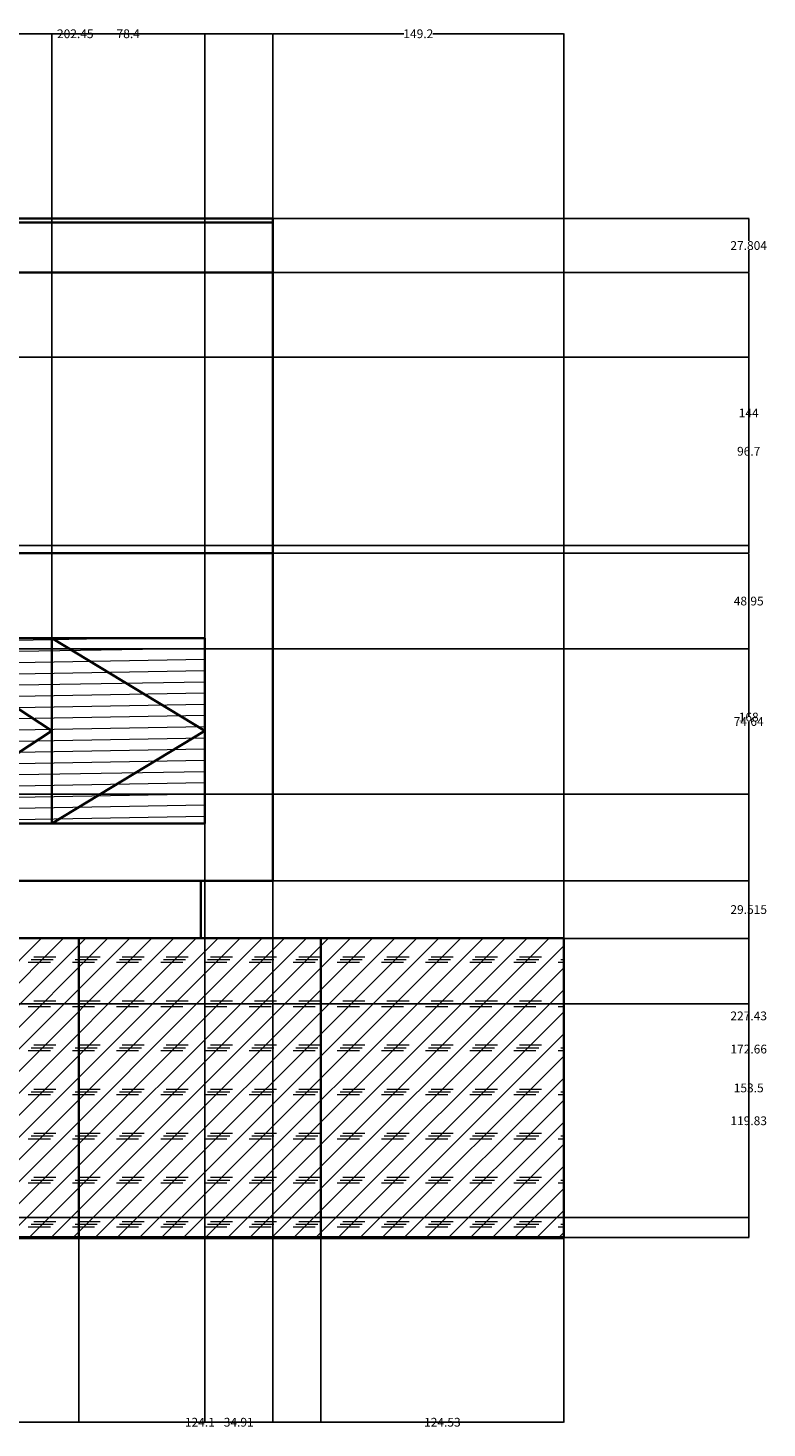
# Model space of a CAD drawing. Units: inches. Extents: x -1308 to 780, y 304 to 1023.
# Tile 7 of 7: x 402 to 780, y 304 to 1023. Entities that reach past the tile are written whole.
import ezdxf

# ---------------------------------------------------------------- set-up
doc = ezdxf.new("R2010")
doc.units = ezdxf.units.IN
doc.header["$MEASUREMENT"] = 0
for name, color, linetype, lineweight in [('A-ANNO-DIMS', 2, 'Continuous', 18), ('A-ELEV', 7, 'Continuous', 35), ('A-ELEV-GRND', 7, 'Continuous', 50), ('A-ELEV-PATT', 8, 'Continuous', 13)]:
    doc.layers.add(name, color=color, linetype=linetype, lineweight=lineweight)
doc.styles.get("Standard").update_dxf_attribs({"font": 'arial.ttf'})
doc.dimstyles.get("Standard").update_dxf_attribs({"dimtxt": 4.5, "dimasz": 0.18, "dimexe": 0.18, "dimexo": 0.0625, "dimgap": 0.09, "dimtad": 0, "dimtih": 1, "dimtoh": 1, "dimdec": 4, "dimzin": 0, "dimdsep": 46, "dimlunit": 4, "dimtxsty": 'Standard', "dimcen": 0.09, "dimadec": 0, "dimazin": 0, "dimtfac": 1, "dimtdec": 4, "dimtofl": 0, "dimtmove": 0, "dimatfit": 3, "dimfxl": 1, "dimtolj": 1, "dimtzin": 0, "dimarcsym": 0})

# ---------------------------------------------------------------- blocks, each defined once
blk = doc.blocks.new('*D1')
at = {"layer": 'A-ANNO-DIMS', "color": 0, "lineweight": -2, "transparency": 16777216}
for p, q in [((-1203.52, 401.95), (-1203.52, 307.09)), ((676.16, 401.95), (676.16, 307.09)), ((-1203.34, 307.27), (-272.9, 307.27)), ((675.98, 307.27), (-254.46, 307.27))]:
    blk.add_line(p, q, dxfattribs=at)
at = {"layer": 'A-ANNO-DIMS', "color": 0, "transparency": 16777216}
for points in [[(-1203.34, 307.3), (-1203.34, 307.24), (-1203.52, 307.27)], [(675.98, 307.3), (675.98, 307.24), (676.16, 307.27)]]:
    blk.add_solid(points, dxfattribs=at)
at = {"layer": 'Defpoints', "color": 0, "transparency": 16777216}
for p in [(-1203.52, 402.02), (676.16, 402.02), (676.16, 307.27)]:
    blk.add_point(p, dxfattribs=at)
at = {"layer": 'A-ANNO-DIMS', "color": 0, "transparency": 16777216, "insert": (-263.68, 307.27), "char_height": 4.5, "attachment_point": 5}
blk.add_mtext('\\A1;1879.7', dxfattribs=at)
blk = doc.blocks.new('*D14')
at = {"layer": 'A-ANNO-DIMS', "color": 0, "lineweight": -2, "transparency": 16777216}
for p, q in [((296.53, 555.46), (296.53, 307.09)), ((427.54, 555.46), (427.54, 307.09)), ((296.71, 307.27), (357.62, 307.27)), ((427.36, 307.27), (366.45, 307.27))]:
    blk.add_line(p, q, dxfattribs=at)
at = {"layer": 'A-ANNO-DIMS', "color": 0, "transparency": 16777216}
for points in [[(296.71, 307.3), (296.71, 307.24), (296.53, 307.27)], [(427.36, 307.3), (427.36, 307.24), (427.54, 307.27)]]:
    blk.add_solid(points, dxfattribs=at)
at = {"layer": 'Defpoints', "color": 0, "transparency": 16777216}
for p in [(296.53, 555.52), (427.54, 555.52), (427.54, 307.27)]:
    blk.add_point(p, dxfattribs=at)
at = {"layer": 'A-ANNO-DIMS', "color": 0, "transparency": 16777216, "insert": (362.03, 307.27), "char_height": 4.5, "attachment_point": 5}
blk.add_mtext('\\A1;131', dxfattribs=at)
blk = doc.blocks.new('*D15')
at = {"layer": 'A-ANNO-DIMS', "color": 0, "lineweight": -2, "transparency": 16777216}
for p, q in [((427.54, 555.46), (427.54, 307.09)), ((551.63, 555.46), (551.63, 307.09)), ((427.72, 307.27), (482.54, 307.27)), ((551.45, 307.27), (496.62, 307.27))]:
    blk.add_line(p, q, dxfattribs=at)
at = {"layer": 'A-ANNO-DIMS', "color": 0, "transparency": 16777216}
for points in [[(427.72, 307.3), (427.72, 307.24), (427.54, 307.27)], [(551.45, 307.3), (551.45, 307.24), (551.63, 307.27)]]:
    blk.add_solid(points, dxfattribs=at)
at = {"layer": 'Defpoints', "color": 0, "transparency": 16777216}
for p in [(427.54, 555.52), (551.63, 555.52), (551.63, 307.27)]:
    blk.add_point(p, dxfattribs=at)
at = {"layer": 'A-ANNO-DIMS', "color": 0, "transparency": 16777216, "insert": (489.58, 307.27), "char_height": 4.5, "attachment_point": 5}
blk.add_mtext('\\A1;124.1', dxfattribs=at)
blk = doc.blocks.new('*D16')
at = {"layer": 'A-ANNO-DIMS', "color": 0, "lineweight": -2, "transparency": 16777216}
for p, q in [((551.63, 555.46), (551.63, 307.09)), ((676.16, 555.46), (676.16, 307.09)), ((551.81, 307.27), (604.67, 307.27)), ((675.98, 307.27), (623.11, 307.27))]:
    blk.add_line(p, q, dxfattribs=at)
at = {"layer": 'A-ANNO-DIMS', "color": 0, "transparency": 16777216}
for points in [[(551.81, 307.3), (551.81, 307.24), (551.63, 307.27)], [(675.98, 307.3), (675.98, 307.24), (676.16, 307.27)]]:
    blk.add_solid(points, dxfattribs=at)
at = {"layer": 'Defpoints', "color": 0, "transparency": 16777216}
for p in [(551.63, 555.52), (676.16, 555.52), (676.16, 307.27)]:
    blk.add_point(p, dxfattribs=at)
at = {"layer": 'A-ANNO-DIMS', "color": 0, "transparency": 16777216, "insert": (613.89, 307.27), "char_height": 4.5, "attachment_point": 5}
blk.add_mtext('\\A1;124.53', dxfattribs=at)
blk = doc.blocks.new('*D18')
at = {"layer": 'A-ANNO-DIMS', "color": 0, "lineweight": -2, "transparency": 16777216}
for p, q in [((-628.68, 924.9), (-628.68, 1019.77)), ((-628.5, 1019.59), (-60.08, 1019.59)), ((526.78, 1019.59), (-41.64, 1019.59)), ((526.96, 924.9), (526.96, 1019.77))]:
    blk.add_line(p, q, dxfattribs=at)
at = {"layer": 'A-ANNO-DIMS', "color": 0, "transparency": 16777216}
for points in [[(-628.5, 1019.62), (-628.5, 1019.56), (-628.68, 1019.59)], [(526.78, 1019.62), (526.78, 1019.56), (526.96, 1019.59)]]:
    blk.add_solid(points, dxfattribs=at)
at = {"layer": 'Defpoints', "color": 0, "transparency": 16777216}
for p in [(526.96, 1019.59), (-628.68, 924.84), (526.96, 924.84)]:
    blk.add_point(p, dxfattribs=at)
at = {"layer": 'A-ANNO-DIMS', "color": 0, "transparency": 16777216, "insert": (-50.86, 1019.59), "char_height": 4.5, "attachment_point": 5}
blk.add_mtext('\\A1;1155.6', dxfattribs=at)
blk = doc.blocks.new('*D19')
at = {"layer": 'A-ANNO-DIMS', "color": 0, "lineweight": -2, "transparency": 16777216}
for p, q in [((526.96, 585.1), (526.96, 1019.77)), ((527.14, 1019.59), (594.11, 1019.59)), ((675.98, 1019.59), (609.01, 1019.59)), ((676.16, 555.59), (676.16, 1019.77))]:
    blk.add_line(p, q, dxfattribs=at)
at = {"layer": 'A-ANNO-DIMS', "color": 0, "transparency": 16777216}
for points in [[(527.14, 1019.62), (527.14, 1019.56), (526.96, 1019.59)], [(675.98, 1019.62), (675.98, 1019.56), (676.16, 1019.59)]]:
    blk.add_solid(points, dxfattribs=at)
at = {"layer": 'Defpoints', "color": 0, "transparency": 16777216}
for p in [(676.16, 1019.59), (526.96, 585.04), (676.16, 555.52)]:
    blk.add_point(p, dxfattribs=at)
at = {"layer": 'A-ANNO-DIMS', "color": 0, "transparency": 16777216, "insert": (601.56, 1019.59), "char_height": 4.5, "attachment_point": 5}
blk.add_mtext('\\A1;149.2', dxfattribs=at)
blk = doc.blocks.new('*D36')
at = {"layer": 'A-ANNO-DIMS', "color": 0, "lineweight": -2, "transparency": 16777216}
for p, q in [((324.51, 753.1), (324.51, 1019.77)), ((324.69, 1019.59), (416.25, 1019.59)), ((526.78, 1019.59), (435.22, 1019.59)), ((526.96, 753.1), (526.96, 1019.77))]:
    blk.add_line(p, q, dxfattribs=at)
at = {"layer": 'A-ANNO-DIMS', "color": 0, "transparency": 16777216}
for points in [[(324.69, 1019.62), (324.69, 1019.56), (324.51, 1019.59)], [(526.78, 1019.62), (526.78, 1019.56), (526.96, 1019.59)]]:
    blk.add_solid(points, dxfattribs=at)
at = {"layer": 'Defpoints', "color": 0, "transparency": 16777216}
for p in [(526.96, 1019.59), (324.51, 753.04), (526.96, 753.04)]:
    blk.add_point(p, dxfattribs=at)
at = {"layer": 'A-ANNO-DIMS', "color": 0, "transparency": 16777216, "insert": (425.73, 1019.59), "char_height": 4.5, "attachment_point": 5}
blk.add_mtext('\\A1;202.45', dxfattribs=at)
blk = doc.blocks.new('*D43')
at = {"layer": 'A-ANNO-DIMS', "color": 0, "lineweight": -2, "transparency": 16777216}
for p, q in [((341.59, 709.52), (341.59, 1019.77)), ((341.77, 1019.59), (369.96, 1019.59)), ((413.47, 1019.59), (385.28, 1019.59)), ((413.65, 709.52), (413.65, 1019.77))]:
    blk.add_line(p, q, dxfattribs=at)
at = {"layer": 'A-ANNO-DIMS', "color": 0, "transparency": 16777216}
for points in [[(341.77, 1019.62), (341.77, 1019.56), (341.59, 1019.59)], [(413.47, 1019.62), (413.47, 1019.56), (413.65, 1019.59)]]:
    blk.add_solid(points, dxfattribs=at)
at = {"layer": 'Defpoints', "color": 0, "transparency": 16777216}
for p in [(413.65, 1019.59), (341.59, 709.46), (413.65, 709.46)]:
    blk.add_point(p, dxfattribs=at)
at = {"layer": 'A-ANNO-DIMS', "color": 0, "transparency": 16777216, "insert": (377.62, 1019.59), "char_height": 4.5, "attachment_point": 5}
blk.add_mtext('\\A1;72.06', dxfattribs=at)
blk = doc.blocks.new('*D44')
at = {"layer": 'A-ANNO-DIMS', "color": 0, "lineweight": -2, "transparency": 16777216}
for p, q in [((413.65, 709.52), (413.65, 1019.77)), ((413.83, 1019.59), (446.95, 1019.59)), ((491.87, 1019.59), (458.76, 1019.59)), ((492.05, 709.52), (492.05, 1019.77))]:
    blk.add_line(p, q, dxfattribs=at)
at = {"layer": 'A-ANNO-DIMS', "color": 0, "transparency": 16777216}
for points in [[(413.83, 1019.62), (413.83, 1019.56), (413.65, 1019.59)], [(491.87, 1019.62), (491.87, 1019.56), (492.05, 1019.59)]]:
    blk.add_solid(points, dxfattribs=at)
at = {"layer": 'Defpoints', "color": 0, "transparency": 16777216}
for p in [(492.05, 1019.59), (413.65, 709.46), (492.05, 709.46)]:
    blk.add_point(p, dxfattribs=at)
at = {"layer": 'A-ANNO-DIMS', "color": 0, "transparency": 16777216, "insert": (452.85, 1019.59), "char_height": 4.5, "attachment_point": 5}
blk.add_mtext('\\A1;78.4', dxfattribs=at)
blk = doc.blocks.new('*D46')
at = {"layer": 'A-ANNO-DIMS', "color": 0, "lineweight": -2, "transparency": 16777216}
for p, q in [((-25.86, 614.44), (-25.86, 307.09)), ((492.05, 614.44), (492.05, 307.09)), ((-25.68, 307.27), (225.41, 307.27)), ((491.87, 307.27), (240.78, 307.27))]:
    blk.add_line(p, q, dxfattribs=at)
at = {"layer": 'A-ANNO-DIMS', "color": 0, "transparency": 16777216}
for points in [[(-25.68, 307.3), (-25.68, 307.24), (-25.86, 307.27)], [(491.87, 307.3), (491.87, 307.24), (492.05, 307.27)]]:
    blk.add_solid(points, dxfattribs=at)
at = {"layer": 'Defpoints', "color": 0, "transparency": 16777216}
for p in [(-25.86, 614.51), (492.05, 614.51), (492.05, 307.27)]:
    blk.add_point(p, dxfattribs=at)
at = {"layer": 'A-ANNO-DIMS', "color": 0, "transparency": 16777216, "insert": (233.1, 307.27), "char_height": 4.5, "attachment_point": 5}
blk.add_mtext('\\A1;517.9', dxfattribs=at)
blk = doc.blocks.new('*D47')
at = {"layer": 'A-ANNO-DIMS', "color": 0, "lineweight": -2, "transparency": 16777216}
for p, q in [((492.05, 614.44), (492.05, 307.09)), ((526.96, 584.98), (526.96, 307.09)), ((492.23, 307.27), (502.26, 307.27)), ((526.78, 307.27), (516.75, 307.27))]:
    blk.add_line(p, q, dxfattribs=at)
at = {"layer": 'A-ANNO-DIMS', "color": 0, "transparency": 16777216}
for points in [[(492.23, 307.3), (492.23, 307.24), (492.05, 307.27)], [(526.78, 307.3), (526.78, 307.24), (526.96, 307.27)]]:
    blk.add_solid(points, dxfattribs=at)
at = {"layer": 'Defpoints', "color": 0, "transparency": 16777216}
for p in [(492.05, 614.51), (526.96, 585.04), (526.96, 307.27)]:
    blk.add_point(p, dxfattribs=at)
at = {"layer": 'A-ANNO-DIMS', "color": 0, "transparency": 16777216, "insert": (509.51, 307.27), "char_height": 4.5, "attachment_point": 5}
blk.add_mtext('\\A1;34.91', dxfattribs=at)
blk = doc.blocks.new('*D58')
at = {"layer": 'A-ANNO-DIMS', "color": 0, "lineweight": -2, "transparency": 16777216}
for p, q in [((-1187.44, 521.84), (771.09, 521.84)), ((770.91, 521.66), (770.91, 464.32)), ((770.91, 402.2), (770.91, 459.54)), ((-1187.44, 402.02), (771.09, 402.02))]:
    blk.add_line(p, q, dxfattribs=at)
at = {"layer": 'A-ANNO-DIMS', "color": 0, "transparency": 16777216}
for points in [[(770.88, 521.66), (770.94, 521.66), (770.91, 521.84)], [(770.88, 402.2), (770.94, 402.2), (770.91, 402.02)]]:
    blk.add_solid(points, dxfattribs=at)
at = {"layer": 'Defpoints', "color": 0, "transparency": 16777216}
for p in [(-1187.5, 521.84), (770.91, 521.84), (-1187.5, 402.02)]:
    blk.add_point(p, dxfattribs=at)
at = {"layer": 'A-ANNO-DIMS', "color": 0, "transparency": 16777216, "insert": (770.91, 461.93), "char_height": 4.5, "attachment_point": 5}
blk.add_mtext('\\A1;119.83', dxfattribs=at)
blk = doc.blocks.new('*D63')
at = {"layer": 'A-ANNO-DIMS', "color": 0, "lineweight": -2, "transparency": 16777216}
for p, q in [((-843.54, 629.44), (771.09, 629.44)), ((770.91, 629.26), (770.91, 518.12)), ((770.91, 402.2), (770.91, 513.34)), ((-843.54, 402.02), (771.09, 402.02))]:
    blk.add_line(p, q, dxfattribs=at)
at = {"layer": 'A-ANNO-DIMS', "color": 0, "transparency": 16777216}
for points in [[(770.88, 629.26), (770.94, 629.26), (770.91, 629.44)], [(770.88, 402.2), (770.94, 402.2), (770.91, 402.02)]]:
    blk.add_solid(points, dxfattribs=at)
at = {"layer": 'Defpoints', "color": 0, "transparency": 16777216}
for p in [(-843.6, 629.44), (770.91, 629.44), (-843.6, 402.02)]:
    blk.add_point(p, dxfattribs=at)
at = {"layer": 'A-ANNO-DIMS', "color": 0, "transparency": 16777216, "insert": (770.91, 515.73), "char_height": 4.5, "attachment_point": 5}
blk.add_mtext('\\A1;227.43', dxfattribs=at)
blk = doc.blocks.new('*D64')
at = {"layer": 'A-ANNO-DIMS', "color": 0, "lineweight": -2, "transparency": 16777216}
for p, q in [((-843.54, 704.09), (771.09, 704.09)), ((770.91, 703.91), (770.91, 669.15)), ((770.91, 629.62), (770.91, 664.38)), ((-843.54, 629.44), (771.09, 629.44))]:
    blk.add_line(p, q, dxfattribs=at)
at = {"layer": 'A-ANNO-DIMS', "color": 0, "transparency": 16777216}
for points in [[(770.88, 703.91), (770.94, 703.91), (770.91, 704.09)], [(770.88, 629.62), (770.94, 629.62), (770.91, 629.44)]]:
    blk.add_solid(points, dxfattribs=at)
at = {"layer": 'Defpoints', "color": 0, "transparency": 16777216}
for p in [(-843.6, 704.09), (770.91, 704.09), (-843.6, 629.44)]:
    blk.add_point(p, dxfattribs=at)
at = {"layer": 'A-ANNO-DIMS', "color": 0, "transparency": 16777216, "insert": (770.91, 666.76), "char_height": 4.5, "attachment_point": 5}
blk.add_mtext('\\A1;74.64', dxfattribs=at)
blk = doc.blocks.new('*D65')
at = {"layer": 'A-ANNO-DIMS', "color": 0, "lineweight": -2, "transparency": 16777216}
for p, q in [((-843.54, 753.04), (771.09, 753.04)), ((770.91, 752.86), (770.91, 730.95)), ((770.91, 704.27), (770.91, 726.17)), ((-843.54, 704.09), (771.09, 704.09))]:
    blk.add_line(p, q, dxfattribs=at)
at = {"layer": 'A-ANNO-DIMS', "color": 0, "transparency": 16777216}
for points in [[(770.88, 752.86), (770.94, 752.86), (770.91, 753.04)], [(770.88, 704.27), (770.94, 704.27), (770.91, 704.09)]]:
    blk.add_solid(points, dxfattribs=at)
at = {"layer": 'Defpoints', "color": 0, "transparency": 16777216}
for p in [(-843.6, 753.04), (770.91, 753.04), (-843.6, 704.09)]:
    blk.add_point(p, dxfattribs=at)
at = {"layer": 'A-ANNO-DIMS', "color": 0, "transparency": 16777216, "insert": (770.91, 728.56), "char_height": 4.5, "attachment_point": 5}
blk.add_mtext('\\A1;48.95', dxfattribs=at)
blk = doc.blocks.new('*D73')
at = {"layer": 'A-ANNO-DIMS', "color": 0, "lineweight": -2, "transparency": 16777216}
for p, q in [((676.22, 555.52), (771.09, 555.52)), ((770.91, 555.34), (770.91, 481.16)), ((770.91, 402.2), (770.91, 476.38)), ((676.22, 402.02), (771.09, 402.02))]:
    blk.add_line(p, q, dxfattribs=at)
at = {"layer": 'A-ANNO-DIMS', "color": 0, "transparency": 16777216}
for points in [[(770.88, 555.34), (770.94, 555.34), (770.91, 555.52)], [(770.88, 402.2), (770.94, 402.2), (770.91, 402.02)]]:
    blk.add_solid(points, dxfattribs=at)
at = {"layer": 'Defpoints', "color": 0, "transparency": 16777216}
for p in [(676.16, 555.52), (770.91, 555.52), (676.16, 402.02)]:
    blk.add_point(p, dxfattribs=at)
at = {"layer": 'A-ANNO-DIMS', "color": 0, "transparency": 16777216, "insert": (770.91, 478.77), "char_height": 4.5, "attachment_point": 5}
blk.add_mtext('\\A1;153.5', dxfattribs=at)
blk = doc.blocks.new('*D74')
at = {"layer": 'A-ANNO-DIMS', "color": 0, "lineweight": -2, "transparency": 16777216}
for p, q in [((527.02, 585.04), (771.09, 585.04)), ((770.91, 584.86), (770.91, 572.67)), ((770.91, 555.7), (770.91, 567.89)), ((676.22, 555.52), (771.09, 555.52))]:
    blk.add_line(p, q, dxfattribs=at)
at = {"layer": 'A-ANNO-DIMS', "color": 0, "transparency": 16777216}
for points in [[(770.88, 584.86), (770.94, 584.86), (770.91, 585.04)], [(770.88, 555.7), (770.94, 555.7), (770.91, 555.52)]]:
    blk.add_solid(points, dxfattribs=at)
at = {"layer": 'Defpoints', "color": 0, "transparency": 16777216}
for p in [(526.96, 585.04), (770.91, 585.04), (676.16, 555.52)]:
    blk.add_point(p, dxfattribs=at)
at = {"layer": 'A-ANNO-DIMS', "color": 0, "transparency": 16777216, "insert": (770.91, 570.28), "char_height": 4.5, "attachment_point": 5}
blk.add_mtext('\\A1;29.515', dxfattribs=at)
blk = doc.blocks.new('*D75')
at = {"layer": 'A-ANNO-DIMS', "color": 0, "lineweight": -2, "transparency": 16777216}
for p, q in [((527.02, 753.04), (771.09, 753.04)), ((770.91, 752.86), (770.91, 671.43)), ((770.91, 585.22), (770.91, 666.65)), ((527.02, 585.04), (771.09, 585.04))]:
    blk.add_line(p, q, dxfattribs=at)
at = {"layer": 'A-ANNO-DIMS', "color": 0, "transparency": 16777216}
for points in [[(770.88, 752.86), (770.94, 752.86), (770.91, 753.04)], [(770.88, 585.22), (770.94, 585.22), (770.91, 585.04)]]:
    blk.add_solid(points, dxfattribs=at)
at = {"layer": 'Defpoints', "color": 0, "transparency": 16777216}
for p in [(526.96, 753.04), (770.91, 753.04), (526.96, 585.04)]:
    blk.add_point(p, dxfattribs=at)
at = {"layer": 'A-ANNO-DIMS', "color": 0, "transparency": 16777216, "insert": (770.91, 669.04), "char_height": 4.5, "attachment_point": 5}
blk.add_mtext('\\A1;168', dxfattribs=at)
blk = doc.blocks.new('*D76')
at = {"layer": 'A-ANNO-DIMS', "color": 0, "lineweight": -2, "transparency": 16777216}
for p, q in [((527.02, 897.04), (771.09, 897.04)), ((770.91, 896.86), (770.91, 827.39)), ((770.91, 753.22), (770.91, 822.69)), ((527.02, 753.04), (771.09, 753.04))]:
    blk.add_line(p, q, dxfattribs=at)
at = {"layer": 'A-ANNO-DIMS', "color": 0, "transparency": 16777216}
for points in [[(770.88, 896.86), (770.94, 896.86), (770.91, 897.04)], [(770.88, 753.22), (770.94, 753.22), (770.91, 753.04)]]:
    blk.add_solid(points, dxfattribs=at)
at = {"layer": 'Defpoints', "color": 0, "transparency": 16777216}
for p in [(526.96, 897.04), (770.91, 897.04), (526.96, 753.04)]:
    blk.add_point(p, dxfattribs=at)
at = {"layer": 'A-ANNO-DIMS', "color": 0, "transparency": 16777216, "insert": (770.91, 825.04), "char_height": 4.5, "attachment_point": 5}
blk.add_mtext('\\A1;144', dxfattribs=at)
blk = doc.blocks.new('*D77')
at = {"layer": 'A-ANNO-DIMS', "color": 0, "lineweight": -2, "transparency": 16777216}
for p, q in [((527.02, 924.84), (771.09, 924.84)), ((770.91, 924.66), (770.91, 913.33)), ((770.91, 897.22), (770.91, 908.55)), ((527.02, 897.04), (771.09, 897.04))]:
    blk.add_line(p, q, dxfattribs=at)
at = {"layer": 'A-ANNO-DIMS', "color": 0, "transparency": 16777216}
for points in [[(770.88, 924.66), (770.94, 924.66), (770.91, 924.84)], [(770.88, 897.22), (770.94, 897.22), (770.91, 897.04)]]:
    blk.add_solid(points, dxfattribs=at)
at = {"layer": 'Defpoints', "color": 0, "transparency": 16777216}
for p in [(526.96, 924.84), (770.91, 924.84), (526.96, 897.04)]:
    blk.add_point(p, dxfattribs=at)
at = {"layer": 'A-ANNO-DIMS', "color": 0, "transparency": 16777216, "insert": (770.91, 910.94), "char_height": 4.5, "attachment_point": 5}
blk.add_mtext('\\A1;27.804', dxfattribs=at)
blk = doc.blocks.new('*D78')
at = {"layer": 'A-ANNO-DIMS', "color": 0, "lineweight": -2, "transparency": 16777216}
for p, q in [((-129.88, 585.04), (771.09, 585.04)), ((770.91, 584.86), (770.91, 501.1)), ((770.91, 412.56), (770.91, 496.32)), ((-129.88, 412.38), (771.09, 412.38))]:
    blk.add_line(p, q, dxfattribs=at)
at = {"layer": 'A-ANNO-DIMS', "color": 0, "transparency": 16777216}
for points in [[(770.88, 584.86), (770.94, 584.86), (770.91, 585.04)], [(770.88, 412.56), (770.94, 412.56), (770.91, 412.38)]]:
    blk.add_solid(points, dxfattribs=at)
at = {"layer": 'Defpoints', "color": 0, "transparency": 16777216}
for p in [(-129.95, 585.04), (770.91, 585.04), (-129.95, 412.38)]:
    blk.add_point(p, dxfattribs=at)
at = {"layer": 'A-ANNO-DIMS', "color": 0, "transparency": 16777216, "insert": (770.91, 498.71), "char_height": 4.5, "attachment_point": 5}
blk.add_mtext('\\A1;172.66', dxfattribs=at)
blk = doc.blocks.new('*D88')
at = {"layer": 'A-ANNO-DIMS', "color": 0, "lineweight": -2, "transparency": 16777216}
for p, q in [((156.98, 853.74), (771.09, 853.74)), ((770.91, 853.56), (770.91, 807.78)), ((770.91, 757.22), (770.91, 803)), ((156.98, 757.04), (771.09, 757.04))]:
    blk.add_line(p, q, dxfattribs=at)
at = {"layer": 'A-ANNO-DIMS', "color": 0, "transparency": 16777216}
for points in [[(770.88, 853.56), (770.94, 853.56), (770.91, 853.74)], [(770.88, 757.22), (770.94, 757.22), (770.91, 757.04)]]:
    blk.add_solid(points, dxfattribs=at)
at = {"layer": 'Defpoints', "color": 0, "transparency": 16777216}
for p in [(156.91, 853.74), (770.91, 853.74), (156.91, 757.04)]:
    blk.add_point(p, dxfattribs=at)
at = {"layer": 'A-ANNO-DIMS', "color": 0, "transparency": 16777216, "insert": (770.91, 805.39), "char_height": 4.5, "attachment_point": 5}
blk.add_mtext('\\A1;96.7', dxfattribs=at)

msp = doc.modelspace()

# ---------------------------------------------------------------- hatches: boundary and pattern name
at = {"layer": 'A-ELEV-PATT'}
h = msp.add_hatch(dxfattribs=at)
h.set_pattern_fill('ANSI31', color=256, scale=46, angle=136)
h.paths.add_polyline_path([(-25.8575, 709.4602), (-25.8575, 614.5069), (31.1601, 661.9835)])
h.paths.add_polyline_path([(31.1601, 709.4602), (-25.8575, 709.4602), (31.1601, 661.9835)], flags=17)
h.paths.add_polyline_path([(31.1601, 661.9835), (-25.8575, 614.5069), (31.1601, 614.5069)])
h.paths.add_polyline_path([(92.9293, 709.4602), (31.1601, 709.4602), (92.9293, 661.9835)])
h.paths.add_polyline_path([(31.1601, 709.4602), (31.1601, 661.9835), (31.1601, 614.5069), (92.9293, 661.9835)])
h.paths.add_polyline_path([(92.9293, 661.9835), (31.1601, 614.5069), (92.9293, 614.5069)])
h.paths.add_polyline_path([(159.4499, 661.9835), (92.9293, 709.4602), (92.9293, 661.9835), (92.9293, 614.5069)])
h.paths.add_polyline_path([(159.4499, 661.9835), (92.9293, 614.5069), (159.4499, 614.5069)])
h.paths.add_polyline_path([(159.4499, 709.4602), (92.9293, 709.4602), (159.4499, 661.9835)], flags=17)
h.paths.add_polyline_path([(159.4499, 709.4602), (159.4499, 614.5069), (221.219, 661.9835)])
h.paths.add_polyline_path([(221.219, 709.4602), (159.4499, 709.4602), (221.219, 661.9835)])
h.paths.add_polyline_path([(221.219, 661.9835), (159.4499, 614.5069), (221.219, 614.5069)])
h.paths.add_polyline_path([(276.6529, 661.9835), (221.219, 709.4602), (221.219, 661.9835), (221.219, 614.5069)])
h.paths.add_polyline_path([(276.6529, 661.9835), (221.219, 614.5069), (276.6529, 614.5069)])
h.paths.add_polyline_path([(276.6529, 709.4602), (221.219, 709.4602), (276.6529, 661.9835)])
h.paths.add_polyline_path([(341.5897, 661.9835), (276.6529, 709.4602), (276.6529, 661.9835), (276.6529, 614.5069)])
h.paths.add_polyline_path([(341.5897, 709.4602), (276.6529, 709.4602), (341.5897, 661.9835)])
h.paths.add_polyline_path([(341.5897, 661.9835), (276.6529, 614.5069), (341.5897, 614.5069)])
h.paths.add_polyline_path([(413.6537, 661.9835), (341.5897, 709.4602), (341.5897, 661.9835), (341.5897, 614.5069)])
h.paths.add_polyline_path([(413.6537, 661.9835), (341.5897, 614.5069), (413.6537, 614.5069)])
h.paths.add_polyline_path([(492.0529, 661.9835), (413.6537, 709.4602), (413.6537, 614.5069)])
h.paths.add_polyline_path([(492.0529, 661.9835), (413.6537, 614.5069), (492.0529, 614.5069)])
h.paths.add_polyline_path([(492.0529, 709.4602), (413.6537, 709.4602), (492.0529, 661.9835)], flags=17)
h.paths.add_polyline_path([(413.6537, 709.4602), (341.5897, 709.4602), (413.6537, 661.9835)])
h = msp.add_hatch(dxfattribs=at)
h.set_pattern_fill('CORK', color=256, scale=64, angle=45)
h.set_pattern_definition([(45, (0, 0), (-5.656854, 5.656854), []), (180, (5.657, 0), (-2e-15, -22.6274), [11.3137, -11.3137]), (180, (7.07, 1.414), (-2e-15, -22.6274), [11.3137, -11.3137]), (180, (8.485, 2.828), (-2e-15, -22.6274), [11.3137, -11.3137])])
h.paths.add_polyline_path([(51.6368, 555.5236), (50.6624, 555.5236), (-59.1597, 555.5236), (-59.1597, 402.0158), (47.1224, 402.0158), (51.6368, 402.0158)])
h.paths.add_polyline_path([(168.0796, 555.5236), (51.6368, 555.5236), (51.6368, 402.0158), (168.0796, 402.0158)])
h.paths.add_polyline_path([(296.5309, 555.5236), (168.0796, 555.5236), (168.0796, 402.0158), (296.5309, 402.0158)])
h.paths.add_polyline_path([(427.5353, 555.5236), (296.5309, 555.5236), (296.5309, 402.0158), (427.5353, 402.0158)])
h.paths.add_polyline_path([(308.7651, 461.4331), (308.7651, 494.0703), (392.3226, 494.0703), (392.3226, 461.4331)], flags=16)
h.paths.add_polyline_path([(310.7651, 463.4331), (310.7651, 492.0703), (390.3226, 492.0703), (390.3226, 463.4331)], flags=0)
h.paths.add_polyline_path([(551.6272, 555.5236), (427.5353, 555.5236), (427.5353, 402.0158), (551.6272, 402.0158)])
h.paths.add_polyline_path([(676.1576, 555.5236), (551.6272, 555.5236), (551.6272, 402.0158), (676.1576, 402.0158), (676.1576, 462.0158)])

# ---------------------------------------------------------------- linework, layer by layer
at = {"layer": 'A-ELEV'}
for p, q in [((381.6743, 924.8421), (526.9606, 924.8421)), ((381.6743, 922.8421), (526.9606, 922.8421)), ((526.9606, 924.8421), (526.9606, 922.8421)), ((526.9606, 922.8421), (526.9606, 897.0385)), ((226.3529, 897.0385), (526.9606, 897.0385)), ((526.9606, 897.0385), (526.9606, 753.0385)), ((526.9606, 753.0385), (-144.7329, 753.0385)), ((526.9606, 585.0385), (526.9606, 753.0385)), ((341.5897, 709.4602), (413.6537, 661.9835)), ((413.6537, 709.4602), (413.6537, 614.5069)), ((413.6537, 709.4602), (492.0529, 661.9835)), ((413.6537, 661.9835), (341.5897, 614.5069)), ((492.0529, 661.9835), (413.6537, 614.5069)), ((-144.7329, 585.0385), (526.9606, 585.0385)), ((490.092, 555.5236), (490.092, 585.0385)), ((676.1576, 555.5236), (50.6624, 555.5236)), ((427.5353, 555.5236), (427.5353, 402.0158)), ((551.6272, 555.5236), (551.6272, 402.0158)), ((676.1576, 462.0158), (676.1576, 555.5236)), ((676.1576, 402.0158), (676.1576, 462.0158))]:
    msp.add_line(p, q, dxfattribs=at)
msp.add_lwpolyline([(-25.8575, 709.4602), (492.0529, 709.4602), (492.0529, 614.5069), (-25.8575, 614.5069)], close=True, dxfattribs=at)
at = {"layer": 'A-ELEV-GRND'}
msp.add_line((47.1224, 402.0158), (676.1576, 402.0158), dxfattribs=at)

# ---------------------------------------------------------------- dimensions: what is measured, and where the dimension line sits
at = {"layer": 'A-ANNO-DIMS'}
for base, p1, p2, override, picture, middle in [((526.9606, 1019.5921), (-628.6809, 924.8421), (526.9606, 924.8421), {"dimdec": 1, "dimlfac": 1, "dimrnd": 0, "dimzin": 0, "dimdsep": 46, "dimlunit": 2}, '*D18', (-50.8601, 1019.5921)), ((526.9606, 1019.5921), (324.5059, 753.0385), (526.9606, 753.0385), {"dimdec": 2, "dimlfac": 1, "dimrnd": 0, "dimzin": 0, "dimdsep": 46, "dimlunit": 2}, '*D36', (425.7333, 1019.5921)), ((413.6537, 1019.5921), (341.5897, 709.4602), (413.6537, 709.4602), {"dimdec": 2, "dimlfac": 1, "dimrnd": 0, "dimzin": 0, "dimdsep": 46, "dimlunit": 2}, '*D43', (377.6217, 1019.5921)), ((492.0529, 1019.5921), (413.6537, 709.4602), (492.0529, 709.4602), {"dimdec": 1, "dimlfac": 1, "dimrnd": 0, "dimzin": 0, "dimdsep": 46, "dimlunit": 2}, '*D44', (452.8533, 1019.5921)), ((676.1576, 1019.5921), (526.9606, 585.0385), (676.1576, 555.5236), {"dimdec": 1, "dimlfac": 1, "dimrnd": 0, "dimzin": 0, "dimdsep": 46, "dimlunit": 2}, '*D19', (601.5591, 1019.5921)), ((492.0529, 307.2658), (-25.8575, 614.5069), (492.0529, 614.5069), {"dimdec": 1, "dimlfac": 1, "dimrnd": 0, "dimzin": 0, "dimdsep": 46, "dimlunit": 2}, '*D46', (233.0977, 307.2658)), ((526.9606, 307.2658), (492.0529, 614.5069), (526.9606, 585.0385), {"dimdec": 2, "dimlfac": 1, "dimrnd": 0, "dimzin": 0, "dimdsep": 46, "dimlunit": 2}, '*D47', (509.5068, 307.2658)), ((427.5353, 307.2658), (296.5309, 555.5236), (427.5353, 555.5236), {"dimdec": 0, "dimlfac": 1, "dimrnd": 0, "dimzin": 0, "dimdsep": 46, "dimlunit": 2}, '*D14', (362.0331, 307.2658)), ((551.6272, 307.2658), (427.5353, 555.5236), (551.6272, 555.5236), {"dimdec": 1, "dimlfac": 1, "dimrnd": 0, "dimzin": 0, "dimdsep": 46, "dimlunit": 2}, '*D15', (489.5812, 307.2658)), ((676.1576, 307.2658), (551.6272, 555.5236), (676.1576, 555.5236), {"dimdec": 2, "dimlfac": 1, "dimrnd": 0, "dimzin": 0, "dimdsep": 46, "dimlunit": 2}, '*D16', (613.8924, 307.2658)), ((676.1576, 307.2658), (-1203.518, 402.0158), (676.1576, 402.0158), {"dimdec": 1, "dimlfac": 1, "dimrnd": 0, "dimzin": 0, "dimdsep": 46, "dimlunit": 2}, '*D1', (-263.6802, 307.2658))]:
    dim = msp.add_linear_dim(base=base, p1=p1, p2=p2, dimstyle='Standard', override=override, dxfattribs=at)
    dim.commit()
    dim.dimension.update_dxf_attribs({"geometry": picture, "text_midpoint": middle})
for base, p1, p2, override, picture, middle in [((770.9076, 924.8421), (526.9606, 897.0385), (526.9606, 924.8421), {"dimdec": 3, "dimlfac": 1, "dimrnd": 0, "dimzin": 0, "dimdsep": 46, "dimlunit": 2}, '*D77', (770.9076, 910.9403)), ((770.9076, 897.0385), (526.9606, 753.0385), (526.9606, 897.0385), {"dimdec": 0, "dimlfac": 1, "dimrnd": 0, "dimzin": 0, "dimdsep": 46, "dimlunit": 2}, '*D76', (770.9076, 825.0385)), ((770.9076, 853.744), (156.9148, 757.0385), (156.9148, 853.744), {"dimdec": 1, "dimlfac": 1, "dimrnd": 0, "dimzin": 0, "dimdsep": 46, "dimlunit": 2}, '*D88', (770.9076, 805.3913)), ((770.9076, 753.0385), (-843.5988, 704.0857), (-843.5988, 753.0385), {"dimdec": 2, "dimlfac": 1, "dimrnd": 0, "dimzin": 0, "dimdsep": 46, "dimlunit": 2}, '*D65', (770.9076, 728.5621)), ((770.9076, 753.0385), (526.9606, 585.0385), (526.9606, 753.0385), {"dimdec": 0, "dimlfac": 1, "dimrnd": 0, "dimzin": 0, "dimdsep": 46, "dimlunit": 2}, '*D75', (770.9076, 669.0385)), ((770.9076, 704.0857), (-843.5988, 629.4421), (-843.5988, 704.0857), {"dimdec": 2, "dimlfac": 1, "dimrnd": 0, "dimzin": 0, "dimdsep": 46, "dimlunit": 2}, '*D64', (770.9076, 666.7639)), ((770.9076, 629.4421), (-843.5988, 402.0158), (-843.5988, 629.4421), {"dimdec": 2, "dimlfac": 1, "dimrnd": 0, "dimzin": 0, "dimdsep": 46, "dimlunit": 2}, '*D63', (770.9076, 515.729)), ((770.9076, 585.0385), (-129.9455, 412.3765), (-129.9455, 585.0385), {"dimdec": 2, "dimlfac": 1, "dimrnd": 0, "dimzin": 0, "dimdsep": 46, "dimlunit": 2}, '*D78', (770.9076, 498.7075)), ((770.9076, 585.0385), (676.1576, 555.5236), (526.9606, 585.0385), {"dimdec": 3, "dimlfac": 1, "dimrnd": 0, "dimzin": 0, "dimdsep": 46, "dimlunit": 2}, '*D74', (770.9076, 570.281)), ((770.9076, 555.5236), (676.1576, 402.0158), (676.1576, 555.5236), {"dimdec": 1, "dimlfac": 1, "dimrnd": 0, "dimzin": 0, "dimdsep": 46, "dimlunit": 2}, '*D73', (770.9076, 478.7697)), ((770.9076, 521.8442), (-1187.498, 402.0158), (-1187.498, 521.8442), {"dimdec": 2, "dimlfac": 1, "dimrnd": 0, "dimzin": 0, "dimdsep": 46, "dimlunit": 2}, '*D58', (770.9076, 461.93))]:
    dim = msp.add_linear_dim(base=base, p1=p1, p2=p2, angle=90, dimstyle='Standard', override=override, dxfattribs=at)
    dim.commit()
    dim.dimension.update_dxf_attribs({"geometry": picture, "text_midpoint": middle})

doc.saveas('drawing.dxf')
